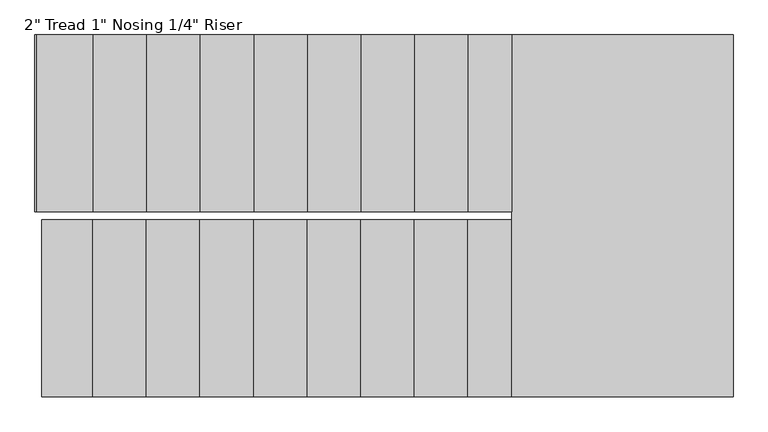
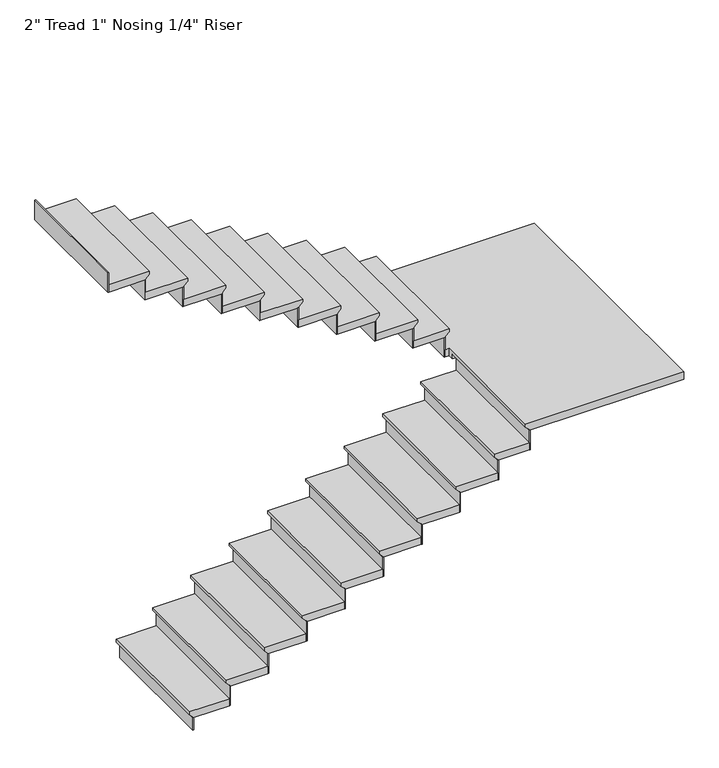
"""IFC4 building model written with IfcOpenShell, lengths in millimetres: stair flight geometry."""

from ifc_helpers import new_model, si_unit, origin, place, context, project, spatial, faceted_brep, source, transform, mapped, element, save


def stair_flight_fbd0abf4(model_context):
    return source(origin(), model_context, "Body", "Brep", [
        faceted_brep([(-1903.1876145, -1606.0595056, 6214.11), (-1903.1876145, -1606.0595056, 6233.16), (-1903.1876145, -767.8595056, 6233.16), (-1903.1876145, -767.8595056, 6214.11), (-1877.7876145, -1606.0595056, 6188.71), (-1877.7876145, -767.8595056, 6188.71), (-1635.543606, -1606.0595056, 6233.16), (-1635.543606, -767.8595056, 6233.16), (-1877.7876145, -767.8595056, 6182.36), (-1635.543606, -767.8595056, 6182.36), (-1635.543606, -1606.0595056, 6182.36), (-1877.7876145, -1606.0595056, 6182.36)], [[[0, 1, 2, 3]], [[4, 0, 3, 5]], [[2, 1, 6, 7]], [[8, 9, 10, 11]], [[2, 7, 9, 8, 5, 3]], [[8, 11, 4, 5]], [[6, 1, 0, 4, 11, 10]], [[7, 6, 10, 9]]]),
        faceted_brep([(-1877.7876145, -1606.0595056, 6182.36), (-1877.7876145, -1606.0595056, 6096.0), (-1871.4376145, -1606.0595056, 6096.0), (-1871.4376145, -1606.0595056, 6182.36), (-1877.7876145, -767.8595056, 6182.36), (-1871.4376145, -767.8595056, 6182.36), (-1871.4376145, -767.8595056, 6096.0), (-1877.7876145, -767.8595056, 6096.0)], [[[0, 1, 2, 3]], [[4, 5, 6, 7]], [[1, 0, 4, 7]], [[2, 1, 7, 6]], [[3, 2, 6, 5]], [[0, 3, 5, 4]]]),
        faceted_brep([(-1635.543606, -1606.0595056, 6319.52), (-1635.543606, -1606.0595056, 6182.36), (-1629.193606, -1606.0595056, 6182.36), (-1629.193606, -1606.0595056, 6319.52), (-1635.543606, -767.8595056, 6319.52), (-1629.193606, -767.8595056, 6319.52), (-1629.193606, -767.8595056, 6182.36), (-1635.543606, -767.8595056, 6182.36)], [[[0, 1, 2, 3]], [[4, 5, 6, 7]], [[1, 0, 4, 7]], [[2, 1, 7, 6]], [[3, 2, 6, 5]], [[0, 3, 5, 4]]]),
        faceted_brep([(-1660.943606, -767.8595056, 6370.32), (-1660.943606, -1606.0595056, 6370.32), (-1381.543606, -1606.0595056, 6370.32), (-1381.543606, -767.8595056, 6370.32), (-1635.543606, -767.8595056, 6319.52), (-1381.543606, -767.8595056, 6319.52), (-1381.543606, -1606.0595056, 6319.52), (-1635.543606, -1606.0595056, 6319.52), (-1635.543606, -767.8595056, 6325.87), (-1660.943606, -767.8595056, 6351.27), (-1635.543606, -1606.0595056, 6325.87), (-1660.943606, -1606.0595056, 6351.27)], [[[0, 1, 2, 3]], [[4, 5, 6, 7]], [[0, 3, 5, 4, 8, 9]], [[4, 7, 10, 8]], [[2, 1, 11, 10, 7, 6]], [[3, 2, 6, 5]], [[11, 1, 0, 9]], [[10, 11, 9, 8]]]),
        faceted_brep([(-1381.543606, -1606.0595056, 6456.68), (-1381.543606, -1606.0595056, 6319.52), (-1375.193606, -1606.0595056, 6319.52), (-1375.193606, -1606.0595056, 6456.68), (-1381.543606, -767.8595056, 6456.68), (-1375.193606, -767.8595056, 6456.68), (-1375.193606, -767.8595056, 6319.52), (-1381.543606, -767.8595056, 6319.52)], [[[0, 1, 2, 3]], [[4, 5, 6, 7]], [[1, 0, 4, 7]], [[2, 1, 7, 6]], [[3, 2, 6, 5]], [[0, 3, 5, 4]]]),
        faceted_brep([(-1406.943606, -767.8595056, 6507.48), (-1406.943606, -1606.0595056, 6507.48), (-1127.543606, -1606.0595056, 6507.48), (-1127.543606, -767.8595056, 6507.48), (-1381.543606, -767.8595056, 6456.68), (-1127.543606, -767.8595056, 6456.68), (-1127.543606, -1606.0595056, 6456.68), (-1381.543606, -1606.0595056, 6456.68), (-1381.543606, -767.8595056, 6463.03), (-1406.943606, -767.8595056, 6488.43), (-1381.543606, -1606.0595056, 6463.03), (-1406.943606, -1606.0595056, 6488.43)], [[[0, 1, 2, 3]], [[4, 5, 6, 7]], [[0, 3, 5, 4, 8, 9]], [[4, 7, 10, 8]], [[2, 1, 11, 10, 7, 6]], [[3, 2, 6, 5]], [[11, 1, 0, 9]], [[10, 11, 9, 8]]]),
        faceted_brep([(-1127.543606, -1606.0595056, 6593.84), (-1127.543606, -1606.0595056, 6456.68), (-1121.193606, -1606.0595056, 6456.68), (-1121.193606, -1606.0595056, 6593.84), (-1127.543606, -767.8595056, 6593.84), (-1121.193606, -767.8595056, 6593.84), (-1121.193606, -767.8595056, 6456.68), (-1127.543606, -767.8595056, 6456.68)], [[[0, 1, 2, 3]], [[4, 5, 6, 7]], [[1, 0, 4, 7]], [[2, 1, 7, 6]], [[3, 2, 6, 5]], [[0, 3, 5, 4]]]),
        faceted_brep([(-1152.943606, -767.8595056, 6644.64), (-1152.943606, -1606.0595056, 6644.64), (-873.543606, -1606.0595056, 6644.64), (-873.543606, -767.8595056, 6644.64), (-1127.543606, -767.8595056, 6593.84), (-873.543606, -767.8595056, 6593.84), (-873.543606, -1606.0595056, 6593.84), (-1127.543606, -1606.0595056, 6593.84), (-1127.543606, -767.8595056, 6600.19), (-1152.943606, -767.8595056, 6625.59), (-1127.543606, -1606.0595056, 6600.19), (-1152.943606, -1606.0595056, 6625.59)], [[[0, 1, 2, 3]], [[4, 5, 6, 7]], [[0, 3, 5, 4, 8, 9]], [[4, 7, 10, 8]], [[2, 1, 11, 10, 7, 6]], [[3, 2, 6, 5]], [[11, 1, 0, 9]], [[10, 11, 9, 8]]]),
        faceted_brep([(-873.543606, -1606.0595056, 6731.0), (-873.543606, -1606.0595056, 6593.84), (-867.193606, -1606.0595056, 6593.84), (-867.193606, -1606.0595056, 6731.0), (-873.543606, -767.8595056, 6731.0), (-867.193606, -767.8595056, 6731.0), (-867.193606, -767.8595056, 6593.84), (-873.543606, -767.8595056, 6593.84)], [[[0, 1, 2, 3]], [[4, 5, 6, 7]], [[1, 0, 4, 7]], [[2, 1, 7, 6]], [[3, 2, 6, 5]], [[0, 3, 5, 4]]]),
        faceted_brep([(-898.943606, -767.8595056, 6781.8), (-898.943606, -1606.0595056, 6781.8), (-619.543606, -1606.0595056, 6781.8), (-619.543606, -767.8595056, 6781.8), (-873.543606, -767.8595056, 6731.0), (-619.543606, -767.8595056, 6731.0), (-619.543606, -1606.0595056, 6731.0), (-873.543606, -1606.0595056, 6731.0), (-873.543606, -767.8595056, 6737.35), (-898.943606, -767.8595056, 6762.75), (-873.543606, -1606.0595056, 6737.35), (-898.943606, -1606.0595056, 6762.75)], [[[0, 1, 2, 3]], [[4, 5, 6, 7]], [[0, 3, 5, 4, 8, 9]], [[4, 7, 10, 8]], [[2, 1, 11, 10, 7, 6]], [[3, 2, 6, 5]], [[11, 1, 0, 9]], [[10, 11, 9, 8]]]),
        faceted_brep([(-619.543606, -1606.0595056, 6868.16), (-619.543606, -1606.0595056, 6731.0), (-613.193606, -1606.0595056, 6731.0), (-613.193606, -1606.0595056, 6868.16), (-619.543606, -767.8595056, 6868.16), (-613.193606, -767.8595056, 6868.16), (-613.193606, -767.8595056, 6731.0), (-619.543606, -767.8595056, 6731.0)], [[[0, 1, 2, 3]], [[4, 5, 6, 7]], [[1, 0, 4, 7]], [[2, 1, 7, 6]], [[3, 2, 6, 5]], [[0, 3, 5, 4]]]),
        faceted_brep([(-644.943606, -767.8595056, 6918.96), (-644.943606, -1606.0595056, 6918.96), (-365.543606, -1606.0595056, 6918.96), (-365.543606, -767.8595056, 6918.96), (-619.543606, -767.8595056, 6868.16), (-365.543606, -767.8595056, 6868.16), (-365.543606, -1606.0595056, 6868.16), (-619.543606, -1606.0595056, 6868.16), (-619.543606, -767.8595056, 6874.51), (-644.943606, -767.8595056, 6899.91), (-619.543606, -1606.0595056, 6874.51), (-644.943606, -1606.0595056, 6899.91)], [[[0, 1, 2, 3]], [[4, 5, 6, 7]], [[0, 3, 5, 4, 8, 9]], [[4, 7, 10, 8]], [[2, 1, 11, 10, 7, 6]], [[3, 2, 6, 5]], [[11, 1, 0, 9]], [[10, 11, 9, 8]]]),
        faceted_brep([(-365.543606, -1606.0595056, 7005.32), (-365.543606, -1606.0595056, 6868.16), (-359.193606, -1606.0595056, 6868.16), (-359.193606, -1606.0595056, 7005.32), (-365.543606, -767.8595056, 7005.32), (-359.193606, -767.8595056, 7005.32), (-359.193606, -767.8595056, 6868.16), (-365.543606, -767.8595056, 6868.16)], [[[0, 1, 2, 3]], [[4, 5, 6, 7]], [[1, 0, 4, 7]], [[2, 1, 7, 6]], [[3, 2, 6, 5]], [[0, 3, 5, 4]]]),
        faceted_brep([(-390.943606, -767.8595056, 7056.12), (-390.943606, -1606.0595056, 7056.12), (-111.543606, -1606.0595056, 7056.12), (-111.543606, -767.8595056, 7056.12), (-365.543606, -767.8595056, 7005.32), (-111.543606, -767.8595056, 7005.32), (-111.543606, -1606.0595056, 7005.32), (-365.543606, -1606.0595056, 7005.32), (-365.543606, -767.8595056, 7011.67), (-390.943606, -767.8595056, 7037.07), (-365.543606, -1606.0595056, 7011.67), (-390.943606, -1606.0595056, 7037.07)], [[[0, 1, 2, 3]], [[4, 5, 6, 7]], [[0, 3, 5, 4, 8, 9]], [[4, 7, 10, 8]], [[2, 1, 11, 10, 7, 6]], [[3, 2, 6, 5]], [[11, 1, 0, 9]], [[10, 11, 9, 8]]]),
        faceted_brep([(-111.543606, -1606.0595056, 7142.48), (-111.543606, -1606.0595056, 7005.32), (-105.193606, -1606.0595056, 7005.32), (-105.193606, -1606.0595056, 7142.48), (-111.543606, -767.8595056, 7142.48), (-105.193606, -767.8595056, 7142.48), (-105.193606, -767.8595056, 7005.32), (-111.543606, -767.8595056, 7005.32)], [[[0, 1, 2, 3]], [[4, 5, 6, 7]], [[1, 0, 4, 7]], [[2, 1, 7, 6]], [[3, 2, 6, 5]], [[0, 3, 5, 4]]]),
        faceted_brep([(-136.943606, -767.8595056, 7193.28), (-136.943606, -1606.0595056, 7193.28), (142.456394, -1606.0595056, 7193.28), (142.456394, -767.8595056, 7193.28), (-111.543606, -767.8595056, 7142.48), (142.456394, -767.8595056, 7142.48), (142.456394, -1606.0595056, 7142.48), (-111.543606, -1606.0595056, 7142.48), (-111.543606, -767.8595056, 7148.83), (-136.943606, -767.8595056, 7174.23), (-111.543606, -1606.0595056, 7148.83), (-136.943606, -1606.0595056, 7174.23)], [[[0, 1, 2, 3]], [[4, 5, 6, 7]], [[0, 3, 5, 4, 8, 9]], [[4, 7, 10, 8]], [[2, 1, 11, 10, 7, 6]], [[3, 2, 6, 5]], [[11, 1, 0, 9]], [[10, 11, 9, 8]]]),
        faceted_brep([(142.456394, -1606.0595056, 7279.64), (142.456394, -1606.0595056, 7142.48), (148.806394, -1606.0595056, 7142.48), (148.806394, -1606.0595056, 7279.64), (142.456394, -767.8595056, 7279.64), (148.806394, -767.8595056, 7279.64), (148.806394, -767.8595056, 7142.48), (142.456394, -767.8595056, 7142.48)], [[[0, 1, 2, 3]], [[4, 5, 6, 7]], [[1, 0, 4, 7]], [[2, 1, 7, 6]], [[3, 2, 6, 5]], [[0, 3, 5, 4]]]),
        faceted_brep([(117.056394, -767.8595056, 7330.44), (117.056394, -1606.0595056, 7330.44), (350.8830625, -1606.0595056, 7330.44), (350.8830625, -767.8595056, 7330.44), (142.456394, -767.8595056, 7279.64), (350.8830625, -767.8595056, 7279.64), (350.8830625, -1606.0595056, 7279.64), (142.456394, -1606.0595056, 7279.64), (142.456394, -767.8595056, 7285.99), (117.056394, -767.8595056, 7311.39), (142.456394, -1606.0595056, 7285.99), (117.056394, -1606.0595056, 7311.39)], [[[0, 1, 2, 3]], [[4, 5, 6, 7]], [[0, 3, 5, 4, 8, 9]], [[4, 7, 10, 8]], [[2, 1, 11, 10, 7, 6]], [[3, 2, 6, 5]], [[11, 1, 0, 9]], [[10, 11, 9, 8]]]),
        faceted_brep([(350.8830625, -1606.0595056, 7416.8), (350.8830625, -1606.0595056, 7279.64), (357.2330625, -1606.0595056, 7279.64), (357.2330625, -1606.0595056, 7416.8), (350.8830625, -767.8595056, 7416.8), (357.2330625, -767.8595056, 7416.8), (357.2330625, -767.8595056, 7279.64), (350.8830625, -767.8595056, 7279.64)], [[[0, 1, 2, 3]], [[4, 5, 6, 7]], [[1, 0, 4, 7]], [[2, 1, 7, 6]], [[3, 2, 6, 5]], [[0, 3, 5, 4]]]),
        faceted_brep([(300.0830625, -729.7595056, 7467.6), (325.4830625, -729.7595056, 7467.6), (325.4830625, -1606.0595056, 7467.6), (1373.4123855, -1606.0595056, 7467.6), (1373.4123855, 108.4404944, 7467.6), (300.0830625, 108.4404944, 7467.6), (325.4830625, -729.7595056, 7416.8), (300.0830625, -729.7595056, 7416.8), (300.0830625, 108.4404944, 7416.8), (1373.4123855, 108.4404944, 7416.8), (1373.4123855, -1606.0595056, 7416.8), (350.8830625, -1606.0595056, 7416.8), (350.8830625, -767.8595056, 7416.8), (325.4830625, -767.8595056, 7416.8), (325.4830625, -767.8595056, 7448.55), (325.4830625, -1606.0595056, 7448.55), (350.8830625, -767.8595056, 7423.15), (350.8830625, -1606.0595056, 7423.15)], [[[0, 1, 2, 3, 4, 5]], [[6, 7, 8, 9, 10, 11, 12, 13]], [[1, 0, 7, 6]], [[2, 1, 6, 13, 14, 15]], [[13, 12, 16, 14]], [[12, 11, 17, 16]], [[3, 2, 15, 17, 11, 10]], [[4, 3, 10, 9]], [[5, 4, 9, 8]], [[0, 5, 8, 7]], [[17, 15, 14, 16]]]),
        faceted_brep([(300.0830625, 108.4404944, 7553.96), (300.0830625, 108.4404944, 7416.8), (293.7330625, 108.4404944, 7416.8), (293.7330625, 108.4404944, 7553.96), (300.0830625, -729.7595056, 7553.96), (293.7330625, -729.7595056, 7553.96), (293.7330625, -729.7595056, 7416.8), (300.0830625, -729.7595056, 7416.8)], [[[0, 1, 2, 3]], [[4, 5, 6, 7]], [[1, 0, 4, 7]], [[2, 1, 7, 6]], [[3, 2, 6, 5]], [[0, 3, 5, 4]]]),
        faceted_brep([(325.4830625, -729.7595056, 7604.76), (325.4830625, 108.4404944, 7604.76), (91.656394, 108.4404944, 7604.76), (91.656394, -729.7595056, 7604.76), (300.0830625, -729.7595056, 7553.96), (91.656394, -729.7595056, 7553.96), (91.656394, 108.4404944, 7553.96), (300.0830625, 108.4404944, 7553.96), (300.0830625, -729.7595056, 7560.31), (325.4830625, -729.7595056, 7585.71), (300.0830625, 108.4404944, 7560.31), (325.4830625, 108.4404944, 7585.71)], [[[0, 1, 2, 3]], [[4, 5, 6, 7]], [[0, 3, 5, 4, 8, 9]], [[4, 7, 10, 8]], [[2, 1, 11, 10, 7, 6]], [[3, 2, 6, 5]], [[11, 1, 0, 9]], [[10, 11, 9, 8]]]),
        faceted_brep([(91.656394, 108.4404944, 7691.12), (91.656394, 108.4404944, 7553.96), (85.306394, 108.4404944, 7553.96), (85.306394, 108.4404944, 7691.12), (91.656394, -729.7595056, 7691.12), (85.306394, -729.7595056, 7691.12), (85.306394, -729.7595056, 7553.96), (91.656394, -729.7595056, 7553.96)], [[[0, 1, 2, 3]], [[4, 5, 6, 7]], [[1, 0, 4, 7]], [[2, 1, 7, 6]], [[3, 2, 6, 5]], [[0, 3, 5, 4]]]),
        faceted_brep([(117.056394, -729.7595056, 7741.92), (117.056394, 108.4404944, 7741.92), (-162.343606, 108.4404944, 7741.92), (-162.343606, -729.7595056, 7741.92), (91.656394, -729.7595056, 7691.12), (-162.343606, -729.7595056, 7691.12), (-162.343606, 108.4404944, 7691.12), (91.656394, 108.4404944, 7691.12), (91.656394, -729.7595056, 7697.47), (117.056394, -729.7595056, 7722.87), (91.656394, 108.4404944, 7697.47), (117.056394, 108.4404944, 7722.87)], [[[0, 1, 2, 3]], [[4, 5, 6, 7]], [[0, 3, 5, 4, 8, 9]], [[4, 7, 10, 8]], [[2, 1, 11, 10, 7, 6]], [[3, 2, 6, 5]], [[11, 1, 0, 9]], [[10, 11, 9, 8]]]),
        faceted_brep([(-162.343606, 108.4404944, 7828.28), (-162.343606, 108.4404944, 7691.12), (-168.693606, 108.4404944, 7691.12), (-168.693606, 108.4404944, 7828.28), (-162.343606, -729.7595056, 7828.28), (-168.693606, -729.7595056, 7828.28), (-168.693606, -729.7595056, 7691.12), (-162.343606, -729.7595056, 7691.12)], [[[0, 1, 2, 3]], [[4, 5, 6, 7]], [[1, 0, 4, 7]], [[2, 1, 7, 6]], [[3, 2, 6, 5]], [[0, 3, 5, 4]]]),
        faceted_brep([(-136.943606, -729.7595056, 7879.08), (-136.943606, 108.4404944, 7879.08), (-416.343606, 108.4404944, 7879.08), (-416.343606, -729.7595056, 7879.08), (-162.343606, -729.7595056, 7828.28), (-416.343606, -729.7595056, 7828.28), (-416.343606, 108.4404944, 7828.28), (-162.343606, 108.4404944, 7828.28), (-162.343606, -729.7595056, 7834.63), (-136.943606, -729.7595056, 7860.03), (-162.343606, 108.4404944, 7834.63), (-136.943606, 108.4404944, 7860.03)], [[[0, 1, 2, 3]], [[4, 5, 6, 7]], [[0, 3, 5, 4, 8, 9]], [[4, 7, 10, 8]], [[2, 1, 11, 10, 7, 6]], [[3, 2, 6, 5]], [[11, 1, 0, 9]], [[10, 11, 9, 8]]]),
        faceted_brep([(-416.343606, 108.4404944, 7965.44), (-416.343606, 108.4404944, 7828.28), (-422.693606, 108.4404944, 7828.28), (-422.693606, 108.4404944, 7965.44), (-416.343606, -729.7595056, 7965.44), (-422.693606, -729.7595056, 7965.44), (-422.693606, -729.7595056, 7828.28), (-416.343606, -729.7595056, 7828.28)], [[[0, 1, 2, 3]], [[4, 5, 6, 7]], [[1, 0, 4, 7]], [[2, 1, 7, 6]], [[3, 2, 6, 5]], [[0, 3, 5, 4]]]),
        faceted_brep([(-390.943606, -729.7595056, 8016.24), (-390.943606, 108.4404944, 8016.24), (-670.343606, 108.4404944, 8016.24), (-670.343606, -729.7595056, 8016.24), (-416.343606, -729.7595056, 7965.44), (-670.343606, -729.7595056, 7965.44), (-670.343606, 108.4404944, 7965.44), (-416.343606, 108.4404944, 7965.44), (-416.343606, -729.7595056, 7971.79), (-390.943606, -729.7595056, 7997.19), (-416.343606, 108.4404944, 7971.79), (-390.943606, 108.4404944, 7997.19)], [[[0, 1, 2, 3]], [[4, 5, 6, 7]], [[0, 3, 5, 4, 8, 9]], [[4, 7, 10, 8]], [[2, 1, 11, 10, 7, 6]], [[3, 2, 6, 5]], [[11, 1, 0, 9]], [[10, 11, 9, 8]]]),
        faceted_brep([(-670.343606, 108.4404944, 8102.6), (-670.343606, 108.4404944, 7965.44), (-676.693606, 108.4404944, 7965.44), (-676.693606, 108.4404944, 8102.6), (-670.343606, -729.7595056, 8102.6), (-676.693606, -729.7595056, 8102.6), (-676.693606, -729.7595056, 7965.44), (-670.343606, -729.7595056, 7965.44)], [[[0, 1, 2, 3]], [[4, 5, 6, 7]], [[1, 0, 4, 7]], [[2, 1, 7, 6]], [[3, 2, 6, 5]], [[0, 3, 5, 4]]]),
        faceted_brep([(-644.943606, -729.7595056, 8153.4), (-644.943606, 108.4404944, 8153.4), (-924.343606, 108.4404944, 8153.4), (-924.343606, -729.7595056, 8153.4), (-670.343606, -729.7595056, 8102.6), (-924.343606, -729.7595056, 8102.6), (-924.343606, 108.4404944, 8102.6), (-670.343606, 108.4404944, 8102.6), (-670.343606, -729.7595056, 8108.95), (-644.943606, -729.7595056, 8134.35), (-670.343606, 108.4404944, 8108.95), (-644.943606, 108.4404944, 8134.35)], [[[0, 1, 2, 3]], [[4, 5, 6, 7]], [[0, 3, 5, 4, 8, 9]], [[4, 7, 10, 8]], [[2, 1, 11, 10, 7, 6]], [[3, 2, 6, 5]], [[11, 1, 0, 9]], [[10, 11, 9, 8]]]),
        faceted_brep([(-924.343606, 108.4404944, 8239.76), (-924.343606, 108.4404944, 8102.6), (-930.693606, 108.4404944, 8102.6), (-930.693606, 108.4404944, 8239.76), (-924.343606, -729.7595056, 8239.76), (-930.693606, -729.7595056, 8239.76), (-930.693606, -729.7595056, 8102.6), (-924.343606, -729.7595056, 8102.6)], [[[0, 1, 2, 3]], [[4, 5, 6, 7]], [[1, 0, 4, 7]], [[2, 1, 7, 6]], [[3, 2, 6, 5]], [[0, 3, 5, 4]]]),
        faceted_brep([(-898.943606, -729.7595056, 8290.56), (-898.943606, 108.4404944, 8290.56), (-1178.343606, 108.4404944, 8290.56), (-1178.343606, -729.7595056, 8290.56), (-924.343606, -729.7595056, 8239.76), (-1178.343606, -729.7595056, 8239.76), (-1178.343606, 108.4404944, 8239.76), (-924.343606, 108.4404944, 8239.76), (-924.343606, -729.7595056, 8246.11), (-898.943606, -729.7595056, 8271.51), (-924.343606, 108.4404944, 8246.11), (-898.943606, 108.4404944, 8271.51)], [[[0, 1, 2, 3]], [[4, 5, 6, 7]], [[0, 3, 5, 4, 8, 9]], [[4, 7, 10, 8]], [[2, 1, 11, 10, 7, 6]], [[3, 2, 6, 5]], [[11, 1, 0, 9]], [[10, 11, 9, 8]]]),
        faceted_brep([(-1178.343606, 108.4404944, 8376.92), (-1178.343606, 108.4404944, 8239.76), (-1184.693606, 108.4404944, 8239.76), (-1184.693606, 108.4404944, 8376.92), (-1178.343606, -729.7595056, 8376.92), (-1184.693606, -729.7595056, 8376.92), (-1184.693606, -729.7595056, 8239.76), (-1178.343606, -729.7595056, 8239.76)], [[[0, 1, 2, 3]], [[4, 5, 6, 7]], [[1, 0, 4, 7]], [[2, 1, 7, 6]], [[3, 2, 6, 5]], [[0, 3, 5, 4]]]),
        faceted_brep([(-1152.943606, -729.7595056, 8427.72), (-1152.943606, 108.4404944, 8427.72), (-1432.343606, 108.4404944, 8427.72), (-1432.343606, -729.7595056, 8427.72), (-1178.343606, -729.7595056, 8376.92), (-1432.343606, -729.7595056, 8376.92), (-1432.343606, 108.4404944, 8376.92), (-1178.343606, 108.4404944, 8376.92), (-1178.343606, -729.7595056, 8383.27), (-1152.943606, -729.7595056, 8408.67), (-1178.343606, 108.4404944, 8383.27), (-1152.943606, 108.4404944, 8408.67)], [[[0, 1, 2, 3]], [[4, 5, 6, 7]], [[0, 3, 5, 4, 8, 9]], [[4, 7, 10, 8]], [[2, 1, 11, 10, 7, 6]], [[3, 2, 6, 5]], [[11, 1, 0, 9]], [[10, 11, 9, 8]]]),
        faceted_brep([(-1432.343606, 108.4404944, 8514.08), (-1432.343606, 108.4404944, 8376.92), (-1438.693606, 108.4404944, 8376.92), (-1438.693606, 108.4404944, 8514.08), (-1432.343606, -729.7595056, 8514.08), (-1438.693606, -729.7595056, 8514.08), (-1438.693606, -729.7595056, 8376.92), (-1432.343606, -729.7595056, 8376.92)], [[[0, 1, 2, 3]], [[4, 5, 6, 7]], [[1, 0, 4, 7]], [[2, 1, 7, 6]], [[3, 2, 6, 5]], [[0, 3, 5, 4]]]),
        faceted_brep([(-1406.943606, -729.7595056, 8564.88), (-1406.943606, 108.4404944, 8564.88), (-1686.343606, 108.4404944, 8564.88), (-1686.343606, -729.7595056, 8564.88), (-1432.343606, -729.7595056, 8514.08), (-1686.343606, -729.7595056, 8514.08), (-1686.343606, 108.4404944, 8514.08), (-1432.343606, 108.4404944, 8514.08), (-1432.343606, -729.7595056, 8520.43), (-1406.943606, -729.7595056, 8545.83), (-1432.343606, 108.4404944, 8520.43), (-1406.943606, 108.4404944, 8545.83)], [[[0, 1, 2, 3]], [[4, 5, 6, 7]], [[0, 3, 5, 4, 8, 9]], [[4, 7, 10, 8]], [[2, 1, 11, 10, 7, 6]], [[3, 2, 6, 5]], [[11, 1, 0, 9]], [[10, 11, 9, 8]]]),
        faceted_brep([(-1686.343606, 108.4404944, 8651.24), (-1686.343606, 108.4404944, 8514.08), (-1692.693606, 108.4404944, 8514.08), (-1692.693606, 108.4404944, 8651.24), (-1686.343606, -729.7595056, 8651.24), (-1692.693606, -729.7595056, 8651.24), (-1692.693606, -729.7595056, 8514.08), (-1686.343606, -729.7595056, 8514.08)], [[[0, 1, 2, 3]], [[4, 5, 6, 7]], [[1, 0, 4, 7]], [[2, 1, 7, 6]], [[3, 2, 6, 5]], [[0, 3, 5, 4]]]),
        faceted_brep([(-1928.5876145, 108.4404944, 8788.4), (-1928.5876145, 108.4404944, 8651.24), (-1934.9376145, 108.4404944, 8651.24), (-1934.9376145, 108.4404944, 8788.4), (-1928.5876145, -729.7595056, 8788.4), (-1934.9376145, -729.7595056, 8788.4), (-1934.9376145, -729.7595056, 8651.24), (-1928.5876145, -729.7595056, 8651.24)], [[[0, 1, 2, 3]], [[4, 5, 6, 7]], [[1, 0, 4, 7]], [[2, 1, 7, 6]], [[3, 2, 6, 5]], [[0, 3, 5, 4]]]),
        faceted_brep([(-1660.943606, -729.7595056, 8702.04), (-1660.943606, 108.4404944, 8702.04), (-1928.5876145, 108.4404944, 8702.04), (-1928.5876145, -729.7595056, 8702.04), (-1686.343606, -729.7595056, 8651.24), (-1928.5876145, -729.7595056, 8651.24), (-1928.5876145, 108.4404944, 8651.24), (-1686.343606, 108.4404944, 8651.24), (-1686.343606, -729.7595056, 8657.59), (-1660.943606, -729.7595056, 8682.99), (-1686.343606, 108.4404944, 8657.59), (-1660.943606, 108.4404944, 8682.99)], [[[0, 1, 2, 3]], [[4, 5, 6, 7]], [[0, 3, 5, 4, 8, 9]], [[4, 7, 10, 8]], [[2, 1, 11, 10, 7, 6]], [[3, 2, 6, 5]], [[11, 1, 0, 9]], [[10, 11, 9, 8]]]),
    ])


if __name__ == "__main__":
    model = new_model("IFC4")
    model_context = context("Model", 3, world=origin())
    ifc_project = project(units=[si_unit("LENGTHUNIT", "METRE", prefix="MILLI")], contexts=[model_context])
    site = spatial("IfcSite", under=ifc_project)
    building = spatial("IfcBuilding", under=site)
    placement = place(None, origin())
    stair_flight_shape = stair_flight_fbd0abf4(model_context)
    element("IfcStairFlight", 1, ObjectType="2\" Tread 1\" Nosing 1/4\" Riser", at=placement, inside=building, context=model_context, shape_type="MappedRepresentation", body=[
        mapped(stair_flight_shape, transform((0.0, 0.0, 0.0), x_axis=(1.0, 0.0, 0.0), y_axis=(0.0, 1.0, 0.0), z_axis=(0.0, 0.0, 1.0))),
    ])
    save(model, "model.ifc")
